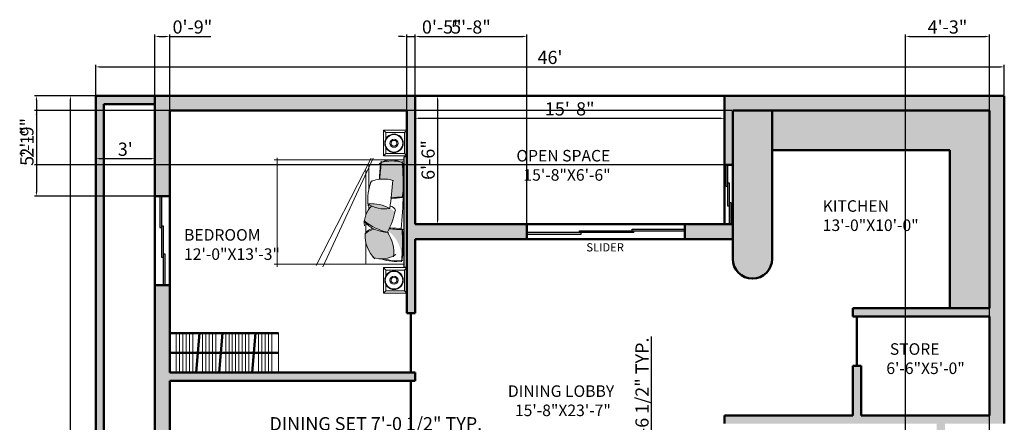
# Model space of a CAD drawing. Units: inches. Extents: x 1913 to 5309, y 1003 to 1733.
# Tile 21 of 23: x 3917 to 4515, y 1489 to 1733. Entities that reach past the tile are written whole.
import ezdxf

# ---------------------------------------------------------------- set-up
doc = ezdxf.new("R2010")
doc.units = ezdxf.units.IN
for name, color, linetype, lineweight in [('0.10', 252, 'Continuous', 9), ('0.15', 34, 'Continuous', 15), ('A-ANNO-DIMS', 2, 'Continuous', 18), ('A-ANNO-TEXT', 7, 'Continuous', 18), ('A-AREA-IDEN', 3, 'Continuous', 18), ('A-FLOR-PATT', 252, 'Continuous', 13), ('A-FURN', 8, 'Continuous', 18), ('A-FURN-PATT', 8, 'Continuous', 13), ('A-GLAZ', 5, 'Continuous', 25), ('A-WALL', 7, 'Continuous', 50)]:
    doc.layers.add(name, color=color, linetype=linetype, lineweight=lineweight)
doc.styles.get("Standard").update_dxf_attribs({"font": 'arial.ttf'})
doc.dimstyles.new('ISO-25', dxfattribs={"dimtxt": 8, "dimasz": 2.5, "dimexe": 1.25, "dimexo": 0.625, "dimtad": 1, "dimdec": 1, "dimlunit": 3, "dimtxsty": 'Standard', "dimcen": 2.5, "dimclrd": 256, "dimclrt": 1, "dimadec": 0, "dimazin": 0, "dimtfac": 1, "dimtdec": 1, "dimtmove": 0, "dimatfit": 3, "dimfxl": 1, "dimarcsym": 0})

# ---------------------------------------------------------------- blocks, each defined once
blk = doc.blocks.new('camita')
at = {"layer": '0.10'}
for p, q in [((-0.85, -0.045), (0.85, -0.045)), ((-0.805, -0.045), (-0.805, -2.048)), ((0.805, -0.045), (0.805, -2.048)), ((-0.827, -0.521), (0.846, -1.293)), ((-0.827, -0.548), (0.824, -1.399)), ((-0.716, -0.585), (-0.355, -0.585)), ((-0.114, -0.585), (-0.049, -0.585)), ((-0.638, -0.63), (0.043, -0.63)), ((0.175, -0.63), (0.318, -0.63)), ((0.474, -0.63), (0.805, -0.63)), ((-0.835, -2), (0.846, -2))]:
    blk.add_line(p, q, dxfattribs=at)
blk.add_lwpolyline([(-0.85, -0.041), (0.85, -0.041), (0.85, 0), (-0.85, 0)], close=True, dxfattribs=at)
for centre, radius, start, end in [((-0.457, -0.236), 0.344, 147.51, 213.8336), ((-0.2, -0.227), 0.586, 163.9263, 197.1409), ((-0.364, -5.846), 5.791, 83.8073, 94.1211), ((-0.51, -1.723), 1.678, 80.1255, 98.6619), ((2.353, -0.053), 2.58, 180.1063, 184.3854), ((-1.544, -0.245), 1.333, 359.9394, 7.5533), ((1.581, -0.289), 1.335, 170.3802, 178.9914), ((-1.44, -0.061), 1.712, 352.9291, 0.3959), ((0.452, -3.067), 3, 83.9026, 93.6759), ((0.486, -1.629), 1.578, 80.1602, 98.06), ((0.029, -0.138), 0.726, 342.5841, 6.0048), ((0.133, -0.17), 0.631, 339.923, 8.7433), ((-0.054, -0.363), 0.454, 159.3026, 206.5026), ((-1.33, -9.675), 9.499, 82.2708, 84.9399), ((0.458, -0.545), 0.584, 151.0456, 184.1497), ((-0.534, -0.339), 0.487, 327.2644, 9.0473), ((-0.007, -0.258), 0.0828, 100.018, 179.736), ((-0.293, -1.438), 1.29, 61.9749, 77.8435), ((-0.199, -0.274), 0.516, 310.7395, 359.0576), ((-0.567, -0.087), 0.906, 321.6953, 346.4626), ((0.627, -0.752), 0.551, 82.9691, 124.6739), ((0.32, -0.394), 0.404, 341.4524, 33.4512), ((-1.867, -14.986), 14.632, 84.6597, 85.7516), ((-0.46, 1.486), 1.909, 260.953, 268.6517), ((-0.2, 0.064), 0.667, 244.7809, 279.0606), ((0.179, -0.272), 0.383, 224.5284, 275.2229), ((0.438, -0.483), 0.19, 193.6849, 236.7035), ((0.571, -0.432), 0.315, 192.9388, 221.9636), ((0.361, -0.133), 0.51, 267.2589, 315.2997)]:
    blk.add_arc(centre, radius, start, end, dxfattribs=at)
blk = doc.blocks.new('VELADOR')
at = {"layer": '0.15'}
for p, q in [((-0.248, 0), (-0.203, -0.045)), ((0.248, 0), (0.202, -0.045)), ((-0.203, -0.405), (-0.248, -0.45)), ((0.248, -0.45), (0.202, -0.405))]:
    blk.add_line(p, q, dxfattribs=at)
blk.add_lwpolyline([(-0.248, 0), (-0.248, -0.45), (0.248, -0.45), (0.248, 0)], close=True, dxfattribs=at)
blk.add_lwpolyline([(0.092, -0.405), (0.202, -0.405), (0.202, -0.045), (-0.203, -0.045), (-0.203, -0.405), (-0.082, -0.405)], dxfattribs=at)
for radius in [0.18, 0.169, 0.0788, 0.0563]:
    blk.add_circle((0.005, -0.247), radius, dxfattribs=at)
blk = doc.blocks.new('*D14')
at = {"layer": 'A-ANNO-DIMS', "color": 0, "lineweight": -2, "transparency": 16777216}
for p, q in [((3962.59, 1686.96), (3946.61, 1686.96)), ((3947.86, 1101.46), (3947.86, 1684.46)), ((3962.59, 1098.96), (3946.61, 1098.96))]:
    blk.add_line(p, q, dxfattribs=at)
at = {"layer": 'A-ANNO-DIMS', "color": 0, "transparency": 16777216}
for points in [[(3947.44, 1684.46), (3948.27, 1684.46), (3947.86, 1686.96)], [(3947.44, 1101.46), (3948.27, 1101.46), (3947.86, 1098.96)]]:
    blk.add_solid(points, dxfattribs=at)
at = {"layer": 'Defpoints', "color": 0, "transparency": 16777216}
for p in [(3947.86, 1686.96), (3963.21, 1686.96), (3963.21, 1098.96)]:
    blk.add_point(p, dxfattribs=at)
at = {"layer": 'A-ANNO-DIMS', "color": 0, "transparency": 16777216, "insert": (3943.15, 1392.96), "char_height": 8, "attachment_point": 5, "rotation": 90}
blk.add_mtext("49'", dxfattribs=at)
blk = doc.blocks.new('*D15')
at = {"layer": 'A-ANNO-DIMS', "color": 0, "lineweight": -2, "transparency": 16777216}
for p, q in [((3963.21, 1687.59), (3963.21, 1705.75)), ((4515.21, 1687.59), (4515.21, 1705.75)), ((3965.71, 1704.5), (4512.71, 1704.5))]:
    blk.add_line(p, q, dxfattribs=at)
at = {"layer": 'A-ANNO-DIMS', "color": 0, "transparency": 16777216}
for points in [[(3965.71, 1704.92), (3965.71, 1704.08), (3963.21, 1704.5)], [(4512.71, 1704.92), (4512.71, 1704.08), (4515.21, 1704.5)]]:
    blk.add_solid(points, dxfattribs=at)
at = {"layer": 'Defpoints', "color": 0, "transparency": 16777216}
for p in [(4515.21, 1704.5), (3963.21, 1686.96), (4515.21, 1686.96)]:
    blk.add_point(p, dxfattribs=at)
at = {"layer": 'A-ANNO-DIMS', "color": 0, "transparency": 16777216, "insert": (4239.21, 1709.21), "char_height": 8, "attachment_point": 5}
blk.add_mtext("46'", dxfattribs=at)
blk = doc.blocks.new('*D16')
at = {"layer": 'A-ANNO-DIMS', "color": 0, "lineweight": -2, "transparency": 16777216}
for p, q in [((4157.21, 1679.78), (4157.21, 1672.02)), ((4345.21, 1679.78), (4345.21, 1672.02)), ((4159.71, 1673.27), (4342.71, 1673.27))]:
    blk.add_line(p, q, dxfattribs=at)
at = {"layer": 'A-ANNO-DIMS', "color": 0, "transparency": 16777216}
for points in [[(4159.71, 1673.68), (4159.71, 1672.85), (4157.21, 1673.27)], [(4342.71, 1673.68), (4342.71, 1672.85), (4345.21, 1673.27)]]:
    blk.add_solid(points, dxfattribs=at)
at = {"layer": 'Defpoints', "color": 0, "transparency": 16777216}
for p in [(4157.21, 1680.41), (4345.21, 1680.41), (4345.21, 1673.27)]:
    blk.add_point(p, dxfattribs=at)
at = {"layer": 'A-ANNO-DIMS', "color": 0, "transparency": 16777216, "insert": (4251.21, 1677.98), "char_height": 8, "attachment_point": 5}
blk.add_mtext('15\'-8"', dxfattribs=at)
blk = doc.blocks.new('*D17')
at = {"layer": 'A-ANNO-DIMS', "color": 0, "lineweight": -2, "transparency": 16777216}
for p, q in [((4171.03, 1686.96), (4169.65, 1686.96)), ((4170.9, 1684.46), (4170.9, 1611.46)), ((4171.03, 1608.96), (4169.65, 1608.96))]:
    blk.add_line(p, q, dxfattribs=at)
at = {"layer": 'A-ANNO-DIMS', "color": 0, "transparency": 16777216}
for points in [[(4170.49, 1684.46), (4171.32, 1684.46), (4170.9, 1686.96)], [(4170.49, 1611.46), (4171.32, 1611.46), (4170.9, 1608.96)]]:
    blk.add_solid(points, dxfattribs=at)
at = {"layer": 'Defpoints', "color": 0, "transparency": 16777216}
for p in [(4171.66, 1686.96), (4170.9, 1608.96), (4171.66, 1608.96)]:
    blk.add_point(p, dxfattribs=at)
at = {"layer": 'A-ANNO-DIMS', "color": 0, "transparency": 16777216, "insert": (4166.19, 1647.96), "char_height": 8, "attachment_point": 5, "rotation": 90}
blk.add_mtext('6\'-6"', dxfattribs=at)
blk = doc.blocks.new('*D38')
at = {"layer": 'A-ANNO-DIMS', "color": 0, "lineweight": -2, "transparency": 16777216}
for p, q in [((3963.21, 1650.65), (3963.21, 1647.53)), ((3996.71, 1648.78), (3965.71, 1648.78)), ((3999.21, 1650.65), (3999.21, 1647.53))]:
    blk.add_line(p, q, dxfattribs=at)
at = {"layer": 'A-ANNO-DIMS', "color": 0, "transparency": 16777216}
for points in [[(3965.71, 1649.19), (3965.71, 1648.36), (3963.21, 1648.78)], [(3996.71, 1649.19), (3996.71, 1648.36), (3999.21, 1648.78)]]:
    blk.add_solid(points, dxfattribs=at)
at = {"layer": 'Defpoints', "color": 0, "transparency": 16777216}
for p in [(3963.21, 1651.28), (3999.21, 1651.28), (3963.21, 1648.78)]:
    blk.add_point(p, dxfattribs=at)
at = {"layer": 'A-ANNO-DIMS', "color": 0, "transparency": 16777216, "insert": (3981.21, 1653.49), "char_height": 8, "attachment_point": 5}
blk.add_mtext("3'", dxfattribs=at)
blk = doc.blocks.new('WIN-54')
for p, q in [((0, 54), (0, 35)), ((1, 54), (1, 17)), ((1, 36), (2, 36)), ((2, 36), (2, 0)), ((0, 35), (1, 35)), ((2, 19), (3, 19)), ((3, 19), (3, 0)), ((1, 17), (2, 17))]:
    blk.add_line(p, q)
blk = doc.blocks.new('WIN-36')
for p, q in [((0, 23), (0, 36)), ((1, 11), (1, 36)), ((2, 25), (1, 25)), ((2, 0), (2, 25)), ((1, 23), (0, 23)), ((3, 13), (2, 13)), ((3, 0), (3, 13)), ((2, 11), (1, 11))]:
    blk.add_line(p, q)
blk = doc.blocks.new('WIN-SLIDER-96')
for p, q in [((65, 1), (0, 1)), ((0, 0), (33, 0)), ((32, 2), (96, 2)), ((32, 1), (32, 2)), ((33, 0), (33, 1)), ((64, 3), (96, 3)), ((64, 2), (64, 3)), ((65, 1), (65, 2))]:
    blk.add_line(p, q)
blk = doc.blocks.new('*D83')
at = {"layer": 'A-ANNO-DIMS', "lineweight": -2, "transparency": 16777216}
for p, q in [((4203.55, 1482.1), (4065.74, 1482.1)), ((4285.72, 1482.1), (4206.05, 1482.1))]:
    blk.add_line(p, q, dxfattribs=at)
at = {"layer": 'A-ANNO-DIMS', "color": 0, "lineweight": -2, "transparency": 16777216}
for p, q in [((4203.55, 1470.03), (4203.55, 1483.35)), ((4288.22, 1470.03), (4288.22, 1483.35))]:
    blk.add_line(p, q, dxfattribs=at)
at = {"layer": 'A-ANNO-DIMS', "transparency": 16777216}
for points in [[(4206.05, 1482.52), (4206.05, 1481.68), (4203.55, 1482.1)], [(4285.72, 1482.52), (4285.72, 1481.68), (4288.22, 1482.1)]]:
    blk.add_solid(points, dxfattribs=at)
at = {"layer": 'Defpoints', "color": 0, "transparency": 16777216}
for p in [(4203.55, 1482.1), (4203.55, 1469.4), (4288.22, 1469.4)]:
    blk.add_point(p, dxfattribs=at)
at = {"layer": 'A-ANNO-DIMS', "color": 1, "transparency": 16777216, "insert": (4133.4, 1486.86), "char_height": 8, "attachment_point": 5}
blk.add_mtext('DINING SET 7\'-0 1/2" TYP.', dxfattribs=at)
blk = doc.blocks.new('*D84')
at = {"layer": 'A-ANNO-DIMS', "lineweight": -2, "transparency": 16777216}
for p, q in [((4300.92, 1469.4), (4300.92, 1540.88)), ((4300.92, 1417.18), (4300.92, 1466.9))]:
    blk.add_line(p, q, dxfattribs=at)
at = {"layer": 'A-ANNO-DIMS', "color": 0, "lineweight": -2, "transparency": 16777216}
for p, q in [((4288.84, 1469.4), (4302.17, 1469.4)), ((4288.84, 1414.68), (4302.17, 1414.68))]:
    blk.add_line(p, q, dxfattribs=at)
at = {"layer": 'A-ANNO-DIMS', "transparency": 16777216}
for points in [[(4300.5, 1466.9), (4301.33, 1466.9), (4300.92, 1469.4)], [(4300.5, 1417.18), (4301.33, 1417.18), (4300.92, 1414.68)]]:
    blk.add_solid(points, dxfattribs=at)
at = {"layer": 'Defpoints', "color": 0, "transparency": 16777216}
for p in [(4288.22, 1469.4), (4300.92, 1469.4), (4288.22, 1414.68)]:
    blk.add_point(p, dxfattribs=at)
at = {"layer": 'A-ANNO-DIMS', "color": 1, "transparency": 16777216, "insert": (4296.16, 1506.39), "char_height": 8, "attachment_point": 5, "rotation": 90}
blk.add_mtext('4\'-6 1/2" TYP.', dxfattribs=at)
blk = doc.blocks.new('*D103')
at = {"layer": 'A-ANNO-DIMS', "color": 0, "lineweight": -2, "transparency": 16777216}
for p, q in [((3999.21, 1687.59), (3999.21, 1724.21)), ((4008.21, 1678.59), (4008.21, 1724.21))]:
    blk.add_line(p, q, dxfattribs=at)
at = {"layer": 'A-ANNO-DIMS', "lineweight": -2, "transparency": 16777216}
for p, q in [((4001.71, 1722.96), (4005.71, 1722.96)), ((4008.21, 1722.96), (4033.23, 1722.96))]:
    blk.add_line(p, q, dxfattribs=at)
at = {"layer": 'A-ANNO-DIMS', "transparency": 16777216}
for points in [[(4001.71, 1723.38), (4001.71, 1722.55), (3999.21, 1722.96)], [(4005.71, 1723.38), (4005.71, 1722.55), (4008.21, 1722.96)]]:
    blk.add_solid(points, dxfattribs=at)
at = {"layer": 'Defpoints', "color": 0, "transparency": 16777216}
for p in [(4008.21, 1722.96), (3999.21, 1686.96), (4008.21, 1677.96)]:
    blk.add_point(p, dxfattribs=at)
at = {"layer": 'A-ANNO-DIMS', "color": 1, "transparency": 16777216, "insert": (4021.97, 1727.67), "char_height": 8, "attachment_point": 5}
blk.add_mtext('0\'-9"', dxfattribs=at)
blk = doc.blocks.new('*D104')
at = {"layer": 'A-ANNO-DIMS', "lineweight": -2, "transparency": 16777216}
for p, q in [((4149.71, 1722.96), (4147.21, 1722.96)), ((4152.21, 1722.96), (4157.21, 1722.96)), ((4159.71, 1722.96), (4184.73, 1722.96))]:
    blk.add_line(p, q, dxfattribs=at)
at = {"layer": 'A-ANNO-DIMS', "color": 0, "lineweight": -2, "transparency": 16777216}
for p, q in [((4152.21, 1678.59), (4152.21, 1724.21)), ((4157.21, 1687.59), (4157.21, 1724.21))]:
    blk.add_line(p, q, dxfattribs=at)
at = {"layer": 'A-ANNO-DIMS', "transparency": 16777216}
for points in [[(4149.71, 1723.38), (4149.71, 1722.55), (4152.21, 1722.96)], [(4159.71, 1723.38), (4159.71, 1722.55), (4157.21, 1722.96)]]:
    blk.add_solid(points, dxfattribs=at)
at = {"layer": 'Defpoints', "color": 0, "transparency": 16777216}
for p in [(4157.21, 1722.96), (4157.21, 1686.96), (4152.21, 1677.96)]:
    blk.add_point(p, dxfattribs=at)
at = {"layer": 'A-ANNO-DIMS', "color": 1, "transparency": 16777216, "insert": (4173.47, 1727.67), "char_height": 8, "attachment_point": 5}
blk.add_mtext('0\'-5"', dxfattribs=at)
blk = doc.blocks.new('*D105')
at = {"layer": 'A-ANNO-DIMS', "color": 0, "lineweight": -2, "transparency": 16777216}
for p, q in [((3998.59, 1686.96), (3925.96, 1686.96)), ((3998.59, 1625.96), (3925.96, 1625.96))]:
    blk.add_line(p, q, dxfattribs=at)
at = {"layer": 'A-ANNO-DIMS', "lineweight": -2, "transparency": 16777216}
blk.add_line((3927.21, 1684.46), (3927.21, 1628.46), dxfattribs=at)
at = {"layer": 'A-ANNO-DIMS', "transparency": 16777216}
for points in [[(3926.8, 1684.46), (3927.63, 1684.46), (3927.21, 1686.96)], [(3926.8, 1628.46), (3927.63, 1628.46), (3927.21, 1625.96)]]:
    blk.add_solid(points, dxfattribs=at)
at = {"layer": 'Defpoints', "color": 0, "transparency": 16777216}
for p in [(3999.21, 1686.96), (3927.21, 1625.96), (3999.21, 1625.96)]:
    blk.add_point(p, dxfattribs=at)
at = {"layer": 'A-ANNO-DIMS', "color": 1, "transparency": 16777216, "insert": (3922.5, 1656.46), "char_height": 8, "attachment_point": 5, "rotation": 90}
blk.add_mtext('5\'-1"', dxfattribs=at)
blk = doc.blocks.new('*D107')
at = {"layer": 'A-ANNO-DIMS', "color": 0, "lineweight": -2, "transparency": 16777216}
for p, q in [((4349.59, 1677.96), (3925.96, 1677.96)), ((4349.59, 1644.96), (3925.96, 1644.96))]:
    blk.add_line(p, q, dxfattribs=at)
at = {"layer": 'A-ANNO-DIMS', "lineweight": -2, "transparency": 16777216}
blk.add_line((3927.21, 1675.46), (3927.21, 1647.46), dxfattribs=at)
at = {"layer": 'A-ANNO-DIMS', "transparency": 16777216}
for points in [[(3926.8, 1675.46), (3927.63, 1675.46), (3927.21, 1677.96)], [(3926.8, 1647.46), (3927.63, 1647.46), (3927.21, 1644.96)]]:
    blk.add_solid(points, dxfattribs=at)
at = {"layer": 'Defpoints', "color": 0, "transparency": 16777216}
for p in [(4350.21, 1677.96), (3927.21, 1644.96), (4350.21, 1644.96)]:
    blk.add_point(p, dxfattribs=at)
at = {"layer": 'A-ANNO-DIMS', "color": 1, "transparency": 16777216, "insert": (3922.5, 1661.46), "char_height": 8, "attachment_point": 5, "rotation": 90}
blk.add_mtext('2\'-9"', dxfattribs=at)
blk = doc.blocks.new('*D108')
at = {"layer": 'A-ANNO-DIMS', "color": 0, "lineweight": -2, "transparency": 16777216}
for p, q in [((4157.21, 1609.59), (4157.21, 1724.21)), ((4225.21, 1609.59), (4225.21, 1724.21))]:
    blk.add_line(p, q, dxfattribs=at)
at = {"layer": 'A-ANNO-DIMS', "lineweight": -2, "transparency": 16777216}
blk.add_line((4159.71, 1722.96), (4222.71, 1722.96), dxfattribs=at)
at = {"layer": 'A-ANNO-DIMS', "transparency": 16777216}
for points in [[(4159.71, 1723.38), (4159.71, 1722.55), (4157.21, 1722.96)], [(4222.71, 1723.38), (4222.71, 1722.55), (4225.21, 1722.96)]]:
    blk.add_solid(points, dxfattribs=at)
at = {"layer": 'Defpoints', "color": 0, "transparency": 16777216}
for p in [(4225.21, 1722.96), (4157.21, 1608.96), (4225.21, 1608.96)]:
    blk.add_point(p, dxfattribs=at)
at = {"layer": 'A-ANNO-DIMS', "color": 1, "transparency": 16777216, "insert": (4191.21, 1727.67), "char_height": 8, "attachment_point": 5}
blk.add_mtext('5\'-8"', dxfattribs=at)
blk = doc.blocks.new('*D113')
at = {"layer": 'A-ANNO-DIMS', "color": 0, "lineweight": -2, "transparency": 16777216}
for p, q in [((4455.21, 1180.59), (4455.21, 1724.21)), ((4506.21, 1180.59), (4506.21, 1724.21))]:
    blk.add_line(p, q, dxfattribs=at)
at = {"layer": 'A-ANNO-DIMS', "lineweight": -2, "transparency": 16777216}
blk.add_line((4457.71, 1722.96), (4503.71, 1722.96), dxfattribs=at)
at = {"layer": 'A-ANNO-DIMS', "transparency": 16777216}
for points in [[(4457.71, 1723.38), (4457.71, 1722.55), (4455.21, 1722.96)], [(4503.71, 1723.38), (4503.71, 1722.55), (4506.21, 1722.96)]]:
    blk.add_solid(points, dxfattribs=at)
at = {"layer": 'Defpoints', "color": 0, "transparency": 16777216}
for p in [(4506.21, 1722.96), (4455.21, 1179.96), (4506.21, 1179.96)]:
    blk.add_point(p, dxfattribs=at)
at = {"layer": 'A-ANNO-DIMS', "color": 1, "transparency": 16777216, "insert": (4480.71, 1727.68), "char_height": 8, "attachment_point": 5}
blk.add_mtext('4\'-3"', dxfattribs=at)

msp = doc.modelspace()

# ---------------------------------------------------------------- hatches: boundary and pattern name
at = {"layer": 'A-FLOR-PATT'}
h = msp.add_hatch(color=256, dxfattribs=at)
h.dxf.hatch_style = 1
h.paths.add_polyline_path([(3968.21, 1681.96), (3999.21, 1681.96), (3999.21, 1686.96), (3963.21, 1686.96), (3963.21, 1098.96), (4008.21, 1098.96), (4008.21, 1103.96), (3968.21, 1103.96)])
h.paths.add_polyline_path([(4515.21, 1146.96), (4510.21, 1146.96), (4510.21, 1103.96), (4128.21, 1103.96), (4128.21, 1098.96), (4515.21, 1098.96)])
h = msp.add_hatch(color=256, dxfattribs=at)
h.dxf.hatch_style = 1
h.paths.add_polyline_path([(4179.21, 1155.93), (4164.35, 1155.93, -0.035946), (4163.9, 1155.96), (4161.21, 1155.96), (4161.21, 1173.96), (4152.21, 1173.96), (4152.21, 1146.96), (4179.21, 1146.96)])
h.paths.add_polyline_path([(4273.21, 1155.96), (4266.93, 1155.96), (4233.21, 1155.96), (4233.21, 1146.96), (4273.21, 1146.96)])
h.paths.add_polyline_path([(4285.21, 1328.96), (4152.21, 1328.96), (4152.21, 1305.96), (4161.21, 1305.96), (4161.21, 1323.96), (4285.21, 1323.96)])
h.paths.add_polyline_path([(4161.21, 1257.96), (4152.21, 1257.96), (4152.21, 1233.96), (4161.21, 1233.96), (4161.21, 1237.71)])
h.paths.add_polyline_path([(4515.21, 1405.96), (4503.21, 1405.96), (4503.21, 1400.96), (4506.21, 1400.96), (4506.21, 1328.96), (4452.21, 1328.96), (4452.21, 1323.96), (4506.21, 1323.96), (4506.21, 1179.96), (4455.21, 1179.96), (4455.21, 1170.96), (4515.21, 1170.96)])
h.paths.add_polyline_path([(4157.21, 1686.96), (3999.21, 1686.96), (3999.21, 1625.96), (4008.21, 1625.96), (4008.21, 1677.96), (4152.21, 1677.96), (4152.21, 1554.96), (4157.21, 1554.96), (4157.21, 1599.96), (4225.21, 1599.96), (4225.21, 1608.96), (4157.21, 1608.96)])
h.paths.add_polyline_path([(4008.21, 1513.96), (4157.21, 1513.96), (4157.21, 1518.96), (4008.21, 1518.96), (4008.21, 1571.96), (3999.21, 1571.96), (3999.21, 1420.96), (4050.21, 1420.96), (4050.21, 1429.96), (4008.21, 1429.96)])
h.paths.add_polyline_path([(4157.21, 1477.96), (4152.21, 1477.96), (4152.21, 1429.96), (4110.21, 1429.96), (4110.21, 1420.96), (4157.21, 1420.96)], flags=17)
h.paths.add_polyline_path([(4350.21, 1608.96), (4345.21, 1608.96), (4321.21, 1608.96), (4321.21, 1599.96), (4350.21, 1599.96)])
h.paths.add_polyline_path([(4515.21, 1686.96), (4345.21, 1686.96), (4345.21, 1644.96), (4350.21, 1644.96), (4350.21, 1677.96), (4506.21, 1677.96), (4506.21, 1557.96), (4423.21, 1557.96), (4423.21, 1552.96), (4506.21, 1552.96), (4506.21, 1492.96), (4428.21, 1492.96), (4428.21, 1522.96), (4423.21, 1522.96), (4423.21, 1492.96), (4345.21, 1492.96), (4345.21, 1487.96), (4474.21, 1487.96), (4474.21, 1464.96), (4479.21, 1464.96), (4479.21, 1487.96), (4515.21, 1487.96)])
h.paths.add_polyline_path([(4479.21, 1428.96), (4474.21, 1428.96), (4474.21, 1405.96), (4345.21, 1405.96), (4345.21, 1358.96), (4350.21, 1358.96), (4350.21, 1400.96), (4417.21, 1400.96), (4417.21, 1394.96), (4422.21, 1394.96), (4422.21, 1400.96), (4479.21, 1400.96)])
h.paths.add_polyline_path([(4350.21, 1323.96), (4422.21, 1323.96), (4422.21, 1370.96), (4417.21, 1370.96), (4417.21, 1328.96), (4345.21, 1328.96), (4345.21, 1158.97, -0.414214), (4342.21, 1155.96), (4327.21, 1155.96), (4327.21, 1146.96), (4350.21, 1146.96), (4350.21, 1170.96), (4401.21, 1170.96), (4401.21, 1179.96), (4350.21, 1179.96)])
h.paths.add_polyline_path([(4157.21, 1356.96), (4152.21, 1356.96), (4152.21, 1352.96), (4157.21, 1352.96)])
h.paths.add_polyline_path([(4157.21, 1396.96), (4152.21, 1396.96), (4152.21, 1392.96), (4157.21, 1392.96)])
h = msp.add_hatch(color=256, dxfattribs=at)
h.dxf.hatch_style = 1
h.paths.add_polyline_path([(4374.21, 1677.96), (4350.21, 1677.96), (4350.21, 1587.96, 1), (4374.21, 1587.96)])
h = msp.add_hatch(color=256, dxfattribs=at)
h.dxf.hatch_style = 1
h.paths.add_polyline_path([(4506.21, 1677.96), (4374.21, 1677.96), (4374.21, 1653.96), (4482.21, 1653.96), (4482.21, 1557.96), (4506.21, 1557.96)])
at = {"layer": 'A-FURN-PATT'}
h = msp.add_hatch(color=256, dxfattribs=at)
h.dxf.hatch_style = 1
h.paths.add_polyline_path([(4135.79, 1636.36, -0.113891), (4143.78, 1635.49, -0.006967), (4142.71, 1625.13, -0.016701), (4149.49, 1625.4, 0.079172), (4149.73, 1646.19, 0.257422), (4136.64, 1646.5, -0.004417)])
h.paths.add_polyline_path([(4149.21, 1589.8, 0.033818), (4149.33, 1605.75, -0.041028), (4138.33, 1606.74, -0.246183)])
h = msp.add_hatch(color=256, dxfattribs=at)
h.dxf.hatch_style = 1
h.paths.add_polyline_path([(4140.45, 1604.13, 0.064806), (4145.06, 1616.41, 0.152135), (4132.31, 1621.36, 0.205841), (4126.51, 1610.96, 0.110131)])
h.paths.add_polyline_path([(4140.54, 1603.99, -0.104045), (4132.44, 1606.06, 0.127326), (4126.93, 1603.2, 0.202559), (4132.32, 1588.54, 0.194952), (4144.21, 1589.82, 0.173835)])

# ---------------------------------------------------------------- linework, layer by layer
at = {"layer": 'A-FURN'}
for p, q in [((4012.21, 1542.96), (4012.21, 1518.96)), ((4014.21, 1542.96), (4014.21, 1518.96)), ((4016.21, 1542.96), (4016.21, 1518.96)), ((4018.21, 1542.96), (4018.21, 1518.96)), ((4020.21, 1542.96), (4020.21, 1518.96)), ((4022.21, 1542.96), (4022.21, 1518.96)), ((4028.21, 1542.96), (4028.21, 1518.96)), ((4030.21, 1542.96), (4030.21, 1518.96)), ((4032.21, 1542.96), (4032.21, 1518.96)), ((4034.21, 1542.96), (4034.21, 1518.96)), ((4036.21, 1542.96), (4036.21, 1518.96)), ((4042.21, 1542.96), (4042.21, 1518.96)), ((4044.21, 1542.96), (4044.21, 1518.96)), ((4046.21, 1542.96), (4046.21, 1518.96)), ((4048.21, 1542.96), (4048.21, 1518.96)), ((4050.21, 1542.96), (4050.21, 1518.96)), ((4052.21, 1542.96), (4052.21, 1518.96)), ((4054.21, 1542.96), (4054.21, 1518.96)), ((4056.21, 1542.96), (4056.21, 1518.96)), ((4062.21, 1542.96), (4062.21, 1518.96)), ((4064.21, 1542.96), (4064.21, 1518.96)), ((4066.21, 1542.96), (4066.21, 1518.96)), ((4068.21, 1542.96), (4068.21, 1518.96)), ((4070.21, 1542.96), (4070.21, 1518.96)), ((4074.21, 1542.96), (4074.21, 1518.96))]:
    msp.add_line(p, q, dxfattribs=at)
at = {"layer": 'A-WALL'}
for p, q in [((3963.21, 1686.96), (4515.21, 1686.96)), ((3963.21, 1098.96), (3963.21, 1686.96)), ((3999.21, 1686.96), (3999.21, 1420.96)), ((4157.21, 1686.96), (4157.21, 1608.96)), ((4345.21, 1686.96), (4345.21, 1608.96)), ((4515.21, 1686.96), (4515.21, 1487.96)), ((3968.21, 1103.96), (3968.21, 1681.96)), ((3968.21, 1681.96), (3999.21, 1681.96)), ((4008.21, 1677.96), (4152.21, 1677.96)), ((4008.21, 1677.96), (4008.21, 1518.96)), ((4152.21, 1677.96), (4152.21, 1554.96)), ((4350.21, 1677.96), (4350.21, 1587.96)), ((4350.21, 1677.96), (4506.21, 1677.96)), ((4374.21, 1677.96), (4374.21, 1587.96)), ((4506.21, 1677.96), (4506.21, 1557.96)), ((4374.21, 1653.96), (4482.21, 1653.96)), ((4482.21, 1653.96), (4482.21, 1557.96)), ((4350.21, 1644.96), (4345.21, 1644.96)), ((3999.21, 1625.96), (4008.21, 1625.96)), ((4157.21, 1608.96), (4345.21, 1608.96)), ((4225.21, 1599.96), (4225.21, 1608.96)), ((4321.21, 1599.96), (4321.21, 1608.96)), ((4350.21, 1608.96), (4345.21, 1608.96)), ((4157.21, 1599.96), (4350.21, 1599.96)), ((4157.21, 1599.96), (4157.21, 1554.96)), ((3999.21, 1571.96), (4008.21, 1571.96)), ((4423.21, 1557.96), (4506.21, 1557.96)), ((4423.21, 1557.96), (4423.21, 1552.96)), ((4152.21, 1554.96), (4157.21, 1554.96)), ((4154.71, 1554.96), (4154.71, 1518.96)), ((4423.21, 1552.96), (4506.21, 1552.96)), ((4425.71, 1522.96), (4425.71, 1552.96)), ((4506.21, 1552.96), (4506.21, 1492.96)), ((4008.21, 1542.96), (4074.21, 1542.96)), ((4026.21, 1542.96), (4024.21, 1518.96)), ((4040.21, 1542.96), (4038.21, 1518.96)), ((4060.21, 1542.96), (4058.21, 1518.96)), ((4074.21, 1530.96), (4008.21, 1530.96)), ((4423.21, 1522.96), (4428.21, 1522.96)), ((4423.21, 1522.96), (4423.21, 1492.96)), ((4428.21, 1522.96), (4428.21, 1492.96)), ((4008.21, 1518.96), (4157.21, 1518.96)), ((4008.21, 1513.96), (4157.21, 1513.96)), ((4008.21, 1513.96), (4008.21, 1429.96)), ((4154.71, 1513.96), (4154.71, 1477.96)), ((4157.21, 1518.96), (4157.21, 1513.96)), ((4345.21, 1492.96), (4423.21, 1492.96)), ((4345.21, 1492.96), (4345.21, 1487.96)), ((4428.21, 1492.96), (4506.21, 1492.96))]:
    msp.add_line(p, q, dxfattribs=at)
msp.add_arc((4362.21, 1587.96), 12, 180, 360, dxfattribs=at)

# ---------------------------------------------------------------- block references
at = {"layer": 'A-FURN'}
for name, p, xscale, yscale, zscale, rotation in [('VELADOR', (4152.21, 1658.3), 31.41542173157097, 31.41542173157097, 31.41542173157097, 270), ('camita', (4152.21, 1616.46), 39.375, 39.375, 39.375, 270), ('VELADOR', (4152.21, 1574.85), -31.41542173157097, 31.41542173157097, 31.41542173157097, 269.9999999999999)]:
    msp.add_blockref(name, p, dxfattribs=dict(at, xscale=xscale, yscale=yscale, zscale=zscale, rotation=rotation))
at = {"layer": 'A-GLAZ'}
for name, p in [('WIN-36', (4346.21, 1608.96)), ('WIN-54', (4002.21, 1571.96)), ('WIN-SLIDER-96', (4225.21, 1602.96))]:
    msp.add_blockref(name, p, dxfattribs=at)

# ---------------------------------------------------------------- texts
at = {"layer": 'A-ANNO-TEXT', "insert": (4261.31, 1597.49), "char_height": 5, "attachment_point": 1}
msp.add_mtext_dynamic_manual_height_columns('{SLIDER}', width=86.9528, gutter_width=12.5, heights=[5.17], dxfattribs=at)
at = {"layer": 'A-AREA-IDEN', "char_height": 7, "attachment_point": 1}
for s, width, insert in [('OPEN SPACE\\P  15\'-8"X6\'-6"', 115.9003, (4218.8, 1654.08)), ('KITCHEN\\P13\'-0"X10\'-0"', 86.9528, (4404.91, 1623.55)), ('BEDROOM\\P12\'-0"X13\'-3"', 86.9528, (4016.89, 1606.02)), (' STORE\\P6\'-6"X5\'-0"', 86.9528, (4443.53, 1536.74)), ('DINING LOBBY\\P  15\'-8"X23\'-7"', 86.9528, (4213.64, 1511.2))]:
    msp.add_mtext_dynamic_manual_height_columns(s, width=width, gutter_width=12.5, heights=[0], dxfattribs=dict(at, insert=insert))

# ---------------------------------------------------------------- dimensions: what is measured, and where the dimension line sits
at = {"layer": 'A-ANNO-DIMS'}
for base, p1, p2, override, picture, middle in [((4008.21, 1722.96), (3999.21, 1686.96), (4008.21, 1677.96), {"dimdec": 1, "dimlfac": 1, "dimrnd": 0, "dimzin": 1, "dimdsep": 46, "dimlunit": 4, "dimfrac": 2}, '*D103', (4021.97, 1727.67)), ((4157.21, 1722.96), (4152.21, 1677.96), (4157.21, 1686.96), {"dimdec": 1, "dimlfac": 1, "dimrnd": 0, "dimzin": 1, "dimdsep": 46, "dimlunit": 4, "dimfrac": 2}, '*D104', (4173.47, 1727.67)), ((4225.21, 1722.96), (4157.21, 1608.96), (4225.21, 1608.96), {"dimdec": 1, "dimlfac": 1, "dimrnd": 0, "dimzin": 1, "dimdsep": 46, "dimlunit": 4, "dimfrac": 2}, '*D108', (4191.21, 1727.67)), ((4506.21, 1722.96), (4455.21, 1179.96), (4506.21, 1179.96), {"dimdec": 1, "dimlfac": 1, "dimrnd": 0, "dimzin": 1, "dimdsep": 46, "dimlunit": 4, "dimfrac": 2}, '*D113', (4480.71, 1727.68)), ((4515.21, 1704.5), (3963.21, 1686.96), (4515.21, 1686.96), {"dimclrd": 0, "dimclre": 0, "dimclrt": 0}, '*D15', (4239.21, 1709.21)), ((4345.21, 1673.27), (4157.21, 1680.41), (4345.21, 1680.41), {"dimclrd": 0, "dimclre": 0, "dimclrt": 0}, '*D16', (4251.21, 1677.98)), ((3963.21, 1648.78), (3999.21, 1651.28), (3963.21, 1651.28), {"dimclrd": 0, "dimclre": 0, "dimclrt": 0}, '*D38', (3981.21, 1653.49))]:
    dim = msp.add_linear_dim(base=base, p1=p1, p2=p2, dimstyle='ISO-25', override=override, dxfattribs=at)
    dim.commit()
    dim.dimension.update_dxf_attribs({"geometry": picture, "text_midpoint": middle})
for base, p1, p2, override, picture, middle in [((3927.21, 1625.96), (3999.21, 1686.96), (3999.21, 1625.96), {"dimdec": 1, "dimlfac": 1, "dimrnd": 0, "dimzin": 1, "dimdsep": 46, "dimlunit": 4, "dimfrac": 2}, '*D105', (3922.5, 1656.46)), ((3947.86, 1686.96), (3963.21, 1098.96), (3963.21, 1686.96), {"dimclrd": 0, "dimclre": 0, "dimclrt": 0}, '*D14', (3943.15, 1392.96)), ((4170.9, 1608.96), (4171.66, 1686.96), (4171.66, 1608.96), {"dimclrd": 0, "dimclre": 0, "dimclrt": 0}, '*D17', (4166.19, 1647.96)), ((3927.21, 1644.96), (4350.21, 1677.96), (4350.21, 1644.96), {"dimdec": 1, "dimlfac": 1, "dimrnd": 0, "dimzin": 1, "dimdsep": 46, "dimlunit": 4, "dimfrac": 2}, '*D107', (3922.5, 1661.46))]:
    dim = msp.add_linear_dim(base=base, p1=p1, p2=p2, angle=90, dimstyle='ISO-25', override=override, dxfattribs=at)
    dim.commit()
    dim.dimension.update_dxf_attribs({"geometry": picture, "text_midpoint": middle})
for base, p1, p2, angle, text, picture, middle in [((4300.92, 1469.4), (4288.22, 1414.68), (4288.22, 1469.4), 90, '<> TYP.', '*D84', (4296.16, 1506.39)), ((4203.55, 1482.1), (4288.22, 1469.4), (4203.55, 1469.4), 180, 'DINING SET <> TYP.', '*D83', (4133.4, 1486.86))]:
    dim = msp.add_linear_dim(base=base, p1=p1, p2=p2, angle=angle, text=text, dimstyle='ISO-25', override={"dimdec": 1, "dimrnd": 0, "dimzin": 1, "dimlunit": 4, "dimfrac": 2}, dxfattribs=at)
    dim.commit()
    dim.dimension.update_dxf_attribs({"geometry": picture, "text_midpoint": middle})

doc.saveas('drawing.dxf')
